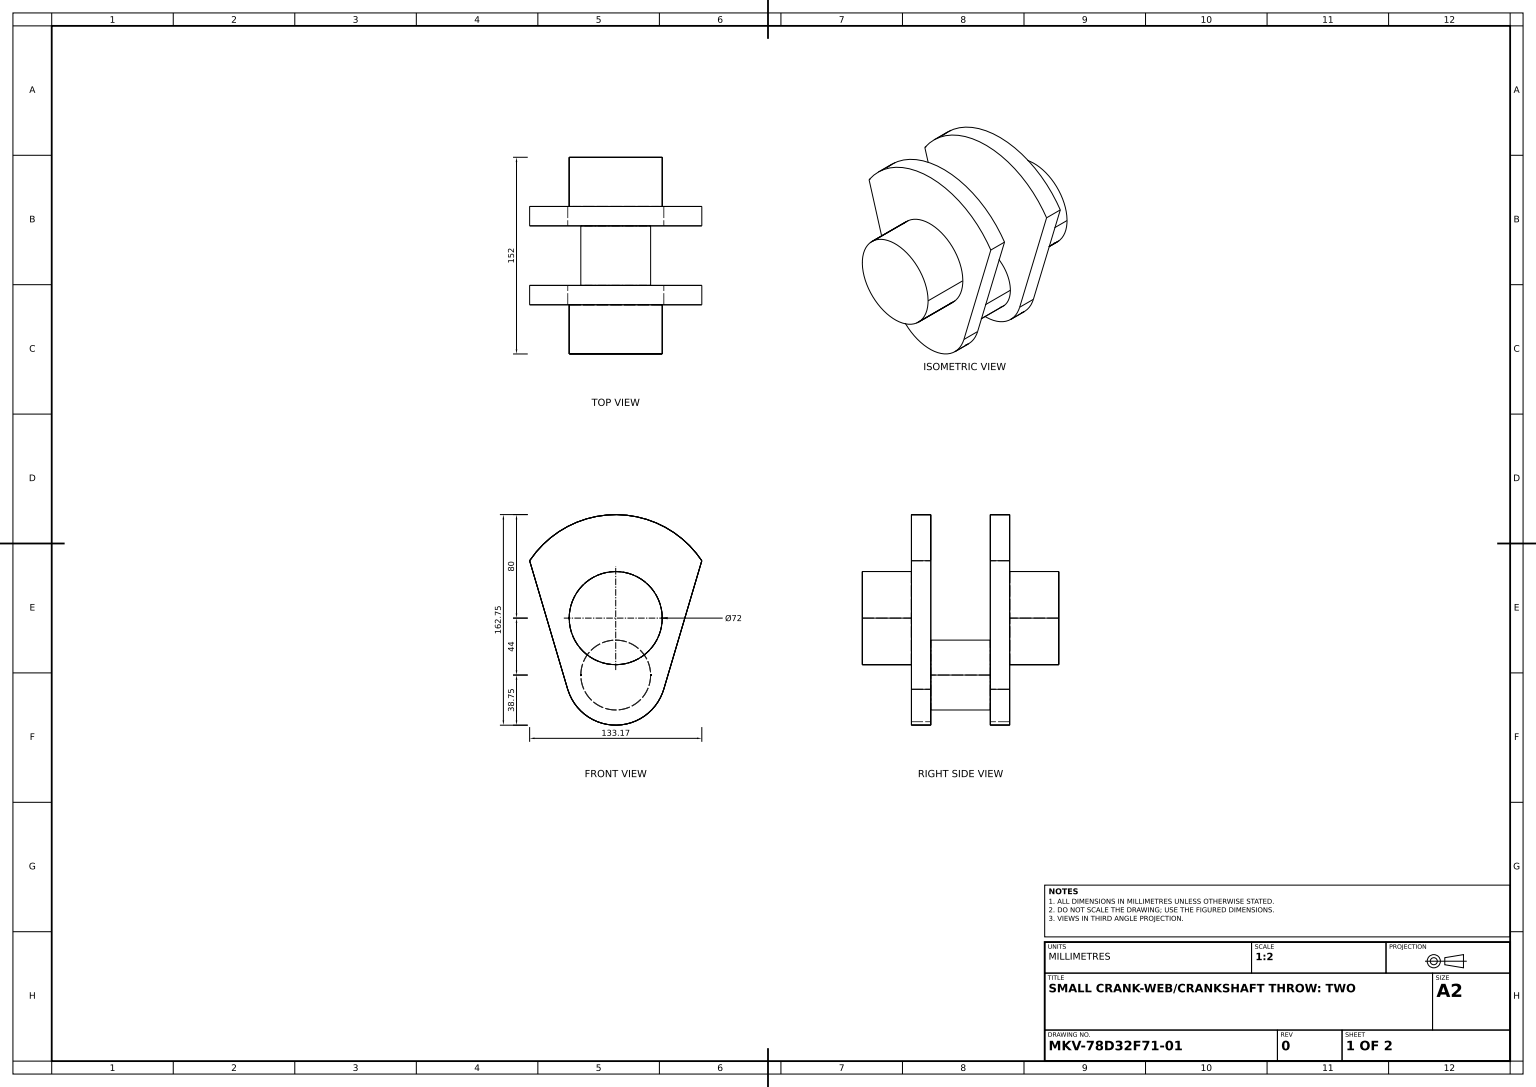
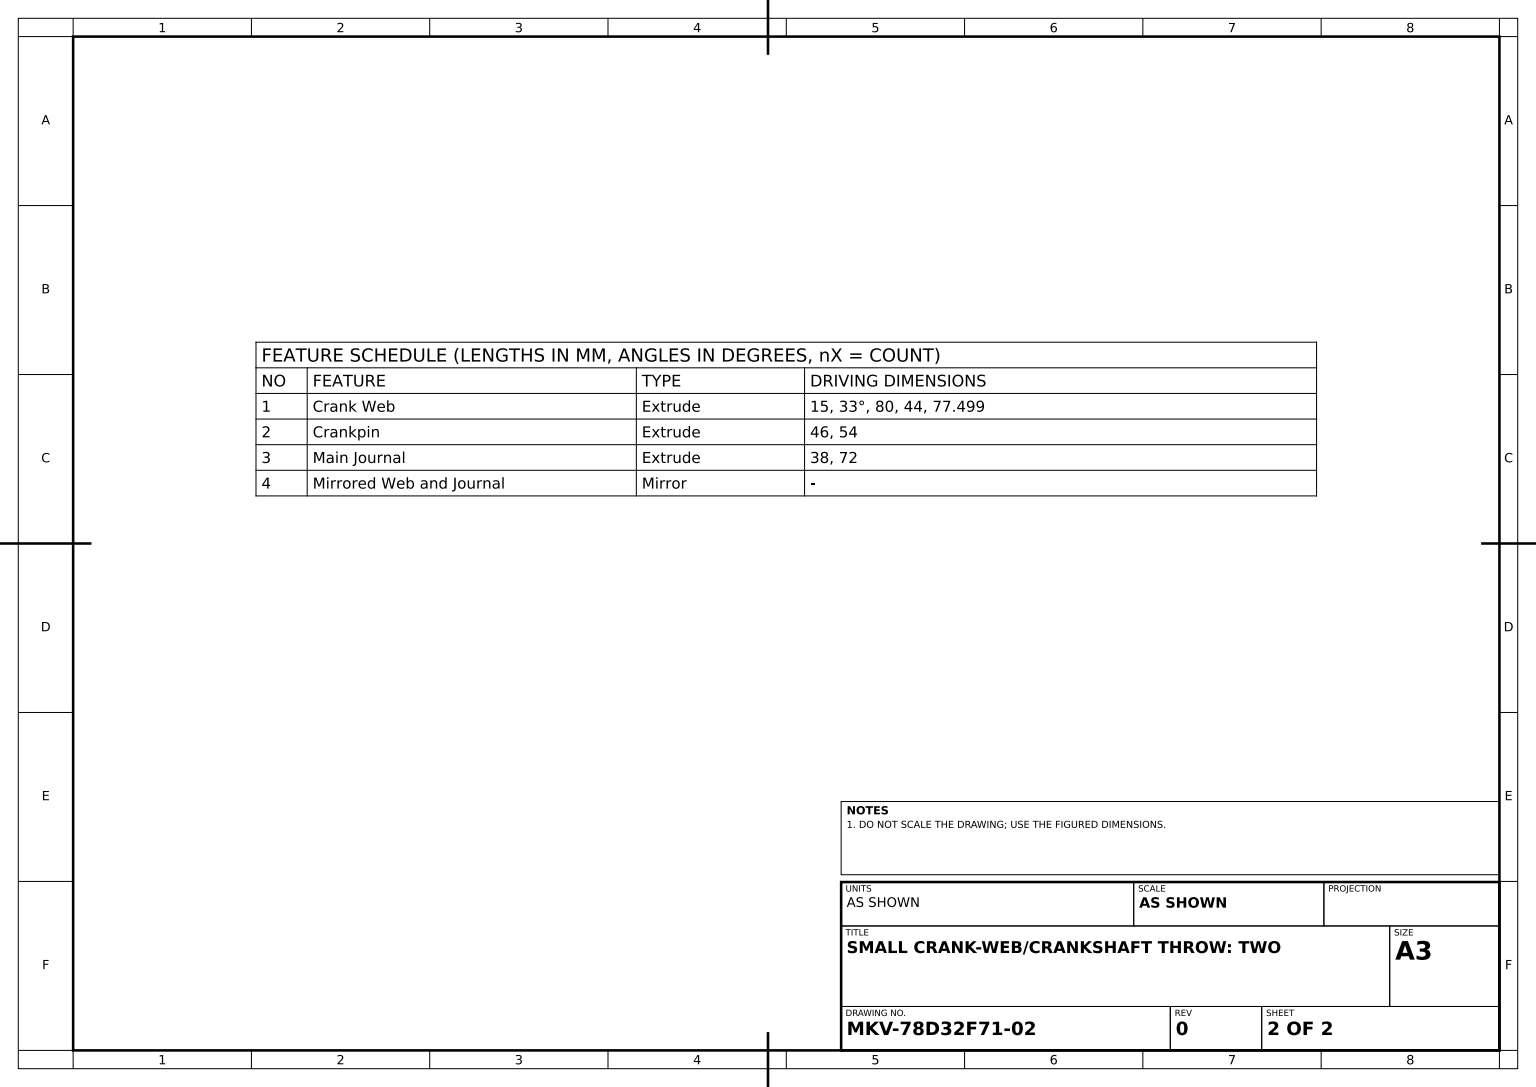
from build123d import *

# Parameters (mm, degrees)
CRANK_WEB_DEPTH        = 15
CRANKPIN_PROFILE_R     = 27
CRANKPIN_DEPTH         = 46
MAIN_JOURNAL_PROFILE_R = 36
MAIN_JOURNAL_DEPTH     = 38


with BuildPart() as part:
    # Crank Web Profile → Crank Web (new body)
    with BuildSketch(Plane.XY):
        with BuildLine():
            ThreePointArc((66.583317356, 44.347061344), (0, 80), (-66.583317356, 44.347061344))
            Line((-66.583317356, 44.347061344), (-37.153763851, -55.005446241))
            ThreePointArc((-37.153763851, -55.005446241), (0, -82.749477613), (37.153763851, -55.005446241))
            Line((37.153763851, -55.005446241), (66.583317356, 44.347061344))
        make_face()
    crank_web = extrude(amount=CRANK_WEB_DEPTH)

    # Crankpin Profile → Crankpin (add)
    with BuildSketch(Plane(origin=(0, 0, 0), x_dir=(-1, 0, 0), z_dir=(0, 0, -1))):
        with Locations(Location((0, -44, 0), (0, 0, 180))):
            Circle(CRANKPIN_PROFILE_R)
    extrude(amount=CRANKPIN_DEPTH)

    # Main Journal Profile → Main Journal (add)
    with BuildSketch(Plane.XY.offset(15)):
        Circle(MAIN_JOURNAL_PROFILE_R)
    main_journal = extrude(amount=MAIN_JOURNAL_DEPTH)

    # Mirrored Web and Journal: Crank Web, Main Journal across plane
    add(crank_web.mirror(Plane(origin=(0, 0, -23), x_dir=(1, 0, 0), z_dir=(0, 0, -1))))
    add(main_journal.mirror(Plane(origin=(0, 0, -23), x_dir=(1, 0, 0), z_dir=(0, 0, -1))))


solid = part.part
